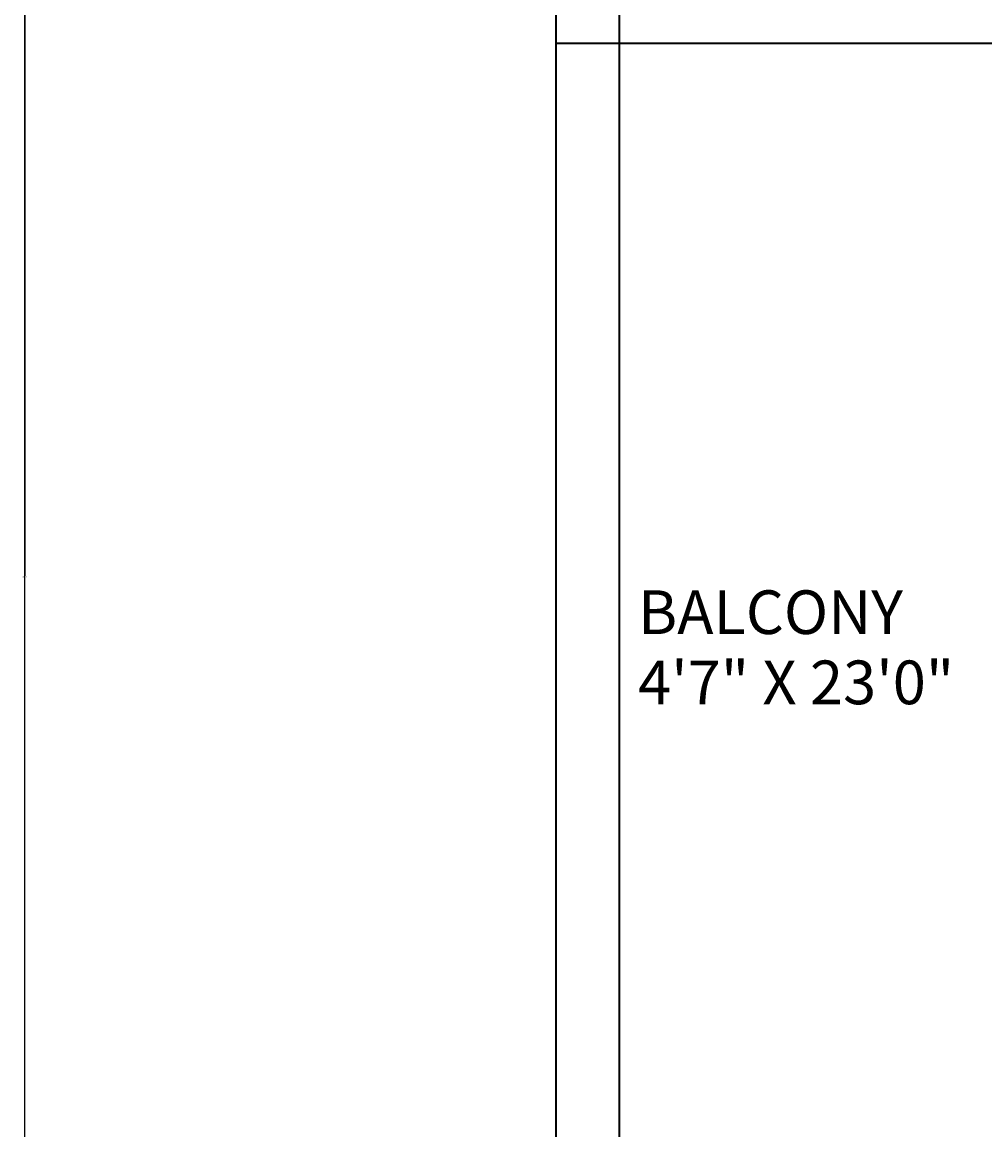
# Model space of a CAD drawing. Units: inches. Extents: x -61 to 1599, y -1316 to 257.
# Tile 13 of 204: x -61 to 76, y -1105 to -947. Entities that reach past the tile are written whole.
import ezdxf

# ---------------------------------------------------------------- set-up
doc = ezdxf.new("R2010")
doc.units = ezdxf.units.IN
doc.header["$MEASUREMENT"] = 0
for name, color, linetype, lineweight in [('A-ANNO-DIMS', 2, 'Continuous', 18), ('A-AREA-IDEN', 1, 'Continuous', 18), ('WALLS', 4, 'Continuous', 35)]:
    doc.layers.add(name, color=color, linetype=linetype, lineweight=lineweight)
doc.styles.get("Standard").update_dxf_attribs({"font": 'arial.ttf'})
doc.dimstyles.get("Standard").update_dxf_attribs({"dimtxt": 0.18, "dimasz": 0.18, "dimexe": 0.18, "dimexo": 0.0625, "dimgap": 0.09, "dimtad": 0, "dimtih": 1, "dimtoh": 1, "dimdec": 0, "dimzin": 0, "dimdsep": 46, "dimlunit": 3, "dimtxsty": 'Standard', "dimcen": 0.09, "dimadec": 0, "dimazin": 0, "dimtfac": 1, "dimtdec": 0, "dimtofl": 0, "dimtmove": 0, "dimatfit": 3, "dimfxl": 1, "dimtolj": 1, "dimtzin": 0, "dimarcsym": 0})

# ---------------------------------------------------------------- blocks, each defined once
blk = doc.blocks.new('*D687')
at = {"layer": 'A-ANNO-DIMS', "color": 0, "lineweight": -2, "transparency": 16777216}
for p, q in [((289.42, 181.68), (-61.08, 181.68)), ((-60.9, 181.5), (-60.9, -528.95)), ((-60.9, -1239.76), (-60.9, -529.32)), ((319.64, -1239.94), (-61.08, -1239.94))]:
    blk.add_line(p, q, dxfattribs=at)
at = {"layer": 'A-ANNO-DIMS', "color": 0, "transparency": 16777216}
for points in [[(-60.93, 181.5), (-60.87, 181.5), (-60.9, 181.68)], [(-60.93, -1239.76), (-60.87, -1239.76), (-60.9, -1239.94)]]:
    blk.add_solid(points, dxfattribs=at)
at = {"layer": 'DEFPOINTS', "color": 0, "transparency": 16777216}
for p in [(289.48, 181.68), (-60.9, -1239.94), (319.7, -1239.94)]:
    blk.add_point(p, dxfattribs=at)
at = {"layer": 'A-ANNO-DIMS', "color": 0, "transparency": 16777216, "insert": (-60.9, -529.13), "char_height": 0.18, "attachment_point": 5}
blk.add_mtext('\\A1;1421.6', dxfattribs=at)
blk = doc.blocks.new('*D693')
at = {"layer": 'A-ANNO-DIMS', "color": 0, "lineweight": -2, "transparency": 16777216}
for p, q in [((14.64, -616.94), (-61.08, -616.94)), ((-60.9, -617.12), (-60.9, -916.26)), ((-60.9, -1215.76), (-60.9, -916.63)), ((14.64, -1215.94), (-61.08, -1215.94))]:
    blk.add_line(p, q, dxfattribs=at)
at = {"layer": 'A-ANNO-DIMS', "color": 0, "transparency": 16777216}
for points in [[(-60.93, -617.12), (-60.87, -617.12), (-60.9, -616.94)], [(-60.93, -1215.76), (-60.87, -1215.76), (-60.9, -1215.94)]]:
    blk.add_solid(points, dxfattribs=at)
at = {"layer": 'DEFPOINTS', "color": 0, "transparency": 16777216}
for p in [(-60.9, -616.94), (14.7, -616.94), (14.7, -1215.94)]:
    blk.add_point(p, dxfattribs=at)
at = {"layer": 'A-ANNO-DIMS', "color": 0, "transparency": 16777216, "insert": (-60.9, -916.44), "char_height": 0.18, "attachment_point": 5}
blk.add_mtext('\\A1;599', dxfattribs=at)
blk = doc.blocks.new('*D696')
at = {"layer": 'A-ANNO-DIMS', "color": 0, "lineweight": -2, "transparency": 16777216}
for p, q in [((690.64, -873.17), (-61.08, -873.17)), ((-60.9, -873.35), (-60.9, -1025.8)), ((-60.9, -1178.61), (-60.9, -1026.16)), ((690.64, -1178.79), (-61.08, -1178.79))]:
    blk.add_line(p, q, dxfattribs=at)
at = {"layer": 'A-ANNO-DIMS', "color": 0, "transparency": 16777216}
for points in [[(-60.93, -873.35), (-60.87, -873.35), (-60.9, -873.17)], [(-60.93, -1178.61), (-60.87, -1178.61), (-60.9, -1178.79)]]:
    blk.add_solid(points, dxfattribs=at)
at = {"layer": 'DEFPOINTS', "color": 0, "transparency": 16777216}
for p in [(-60.9, -873.17), (690.7, -873.17), (690.7, -1178.79)]:
    blk.add_point(p, dxfattribs=at)
at = {"layer": 'A-ANNO-DIMS', "color": 0, "transparency": 16777216, "insert": (-60.9, -1025.98), "char_height": 0.18, "attachment_point": 5}
blk.add_mtext('\\A1;305.6', dxfattribs=at)

msp = doc.modelspace()

# ---------------------------------------------------------------- linework, layer by layer
at = {"layer": 'WALLS'}
for p, q in [((14.7028, -616.9446), (14.7028, -1215.9446)), ((23.7028, -943.9446), (23.7028, -1215.9446)), ((14.7028, -949.9446), (234.7028, -949.9446))]:
    msp.add_line(p, q, dxfattribs=at)

# ---------------------------------------------------------------- texts
at = {"layer": 'A-AREA-IDEN'}
for s, height, p in [('BALCONY', 6.22364, (26.4051, -1034.1012)), ('4\'7" X 23\'0"', 6.223643, (26.4051, -1044.0989))]:
    msp.add_text(s, height=height, dxfattribs=at).set_placement(p)

# ---------------------------------------------------------------- dimensions: what is measured, and where the dimension line sits
at = {"layer": 'A-ANNO-DIMS'}
for base, p1, p2, override, picture, middle in [((-60.8972, -1239.9446), (289.4807, 181.6771), (319.7028, -1239.9446), {"dimdec": 1, "dimlfac": 1, "dimrnd": 0, "dimzin": 0, "dimdsep": 46, "dimlunit": 2}, '*D687', (-60.8972, -529.1337)), ((-60.8972, -616.9446), (14.7028, -1215.9446), (14.7028, -616.9446), {"dimdec": 0, "dimlfac": 1, "dimrnd": 0, "dimzin": 0, "dimdsep": 46, "dimlunit": 2}, '*D693', (-60.8972, -916.4446)), ((-60.8972, -873.169), (690.7028, -1178.7933), (690.7028, -873.169), {"dimdec": 1, "dimlfac": 1, "dimrnd": 0, "dimzin": 0, "dimdsep": 46, "dimlunit": 2}, '*D696', (-60.8972, -1025.9812))]:
    dim = msp.add_linear_dim(base=base, p1=p1, p2=p2, angle=90, dimstyle='Standard', override=override, dxfattribs=at)
    dim.commit()
    dim.dimension.update_dxf_attribs({"geometry": picture, "text_midpoint": middle})

doc.saveas('drawing.dxf')
